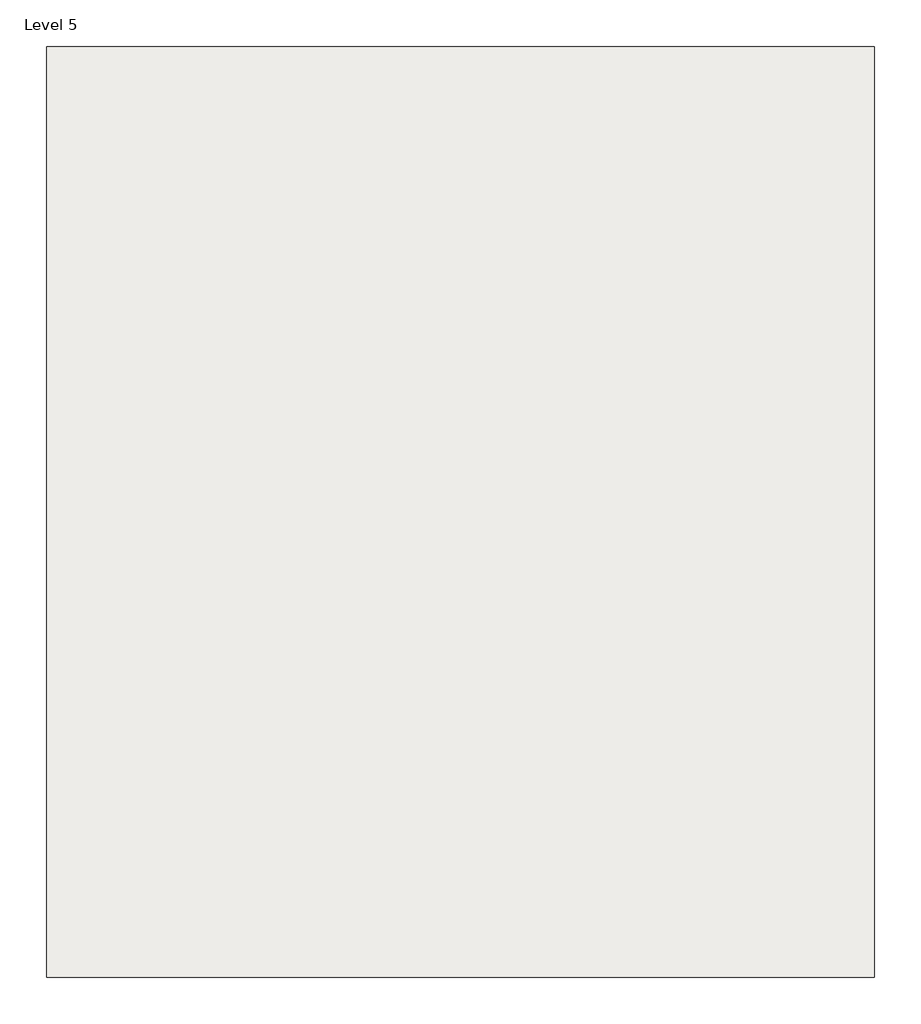
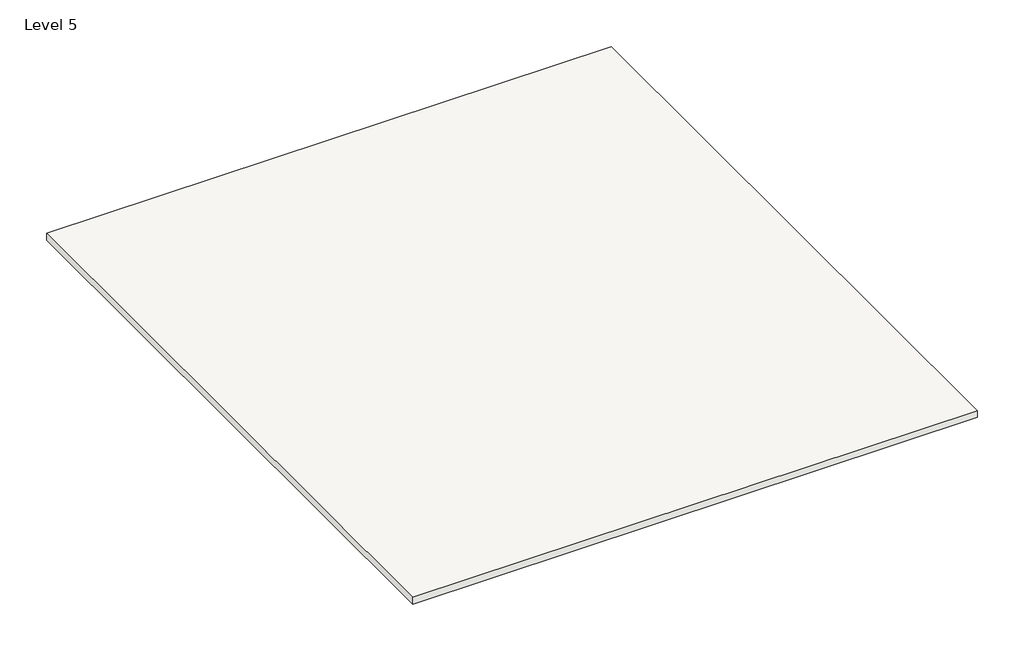
# One storey, incomplete: 1 roof.
"""IFC4 building model written with IfcOpenShell, lengths in millimetres."""

from ifc_helpers import new_model, si_unit, frame, origin, place, context, project, spatial, polyline, outline, extrude, element, save

model = new_model("IFC4")

# Units and contexts
model_context = context("Model", 3, world=origin())
ifc_project = project(units=[si_unit("LENGTHUNIT", "METRE", prefix="MILLI")], contexts=[model_context])

# Site, building, storey
site = spatial("IfcSite", under=ifc_project)
building = spatial("IfcBuilding", under=site)
storey = spatial("IfcBuildingStorey", under=building, Name="Level 5", Elevation=12192.0)

# Roof
placement = place(None, origin())
element("IfcRoof", 1, ObjectType="Generic - 12\"", at=placement, inside=storey, context=model_context, shape_type="SweptSolid", body=[
    extrude(outline(polyline([(-6906.5690281, 7421.1495467), (5272.7309719, 7421.1495467), (5272.7309719, -6269.4504533), (-6906.5690281, -6269.4504533), (-6906.5690281, 7421.1495467)])), frame((0.0, 0.0, 12192.0), z_axis=(0.0, 0.0, 1.0), x_axis=(1.0, 0.0, 0.0)), (0.0, 0.0, 1.0), 152.4),
])

save(model, "model.ifc")

# Revit data of these elements
# Type "Generic - 12\""
#   Assembly Code = "B1020"
#   Layers, outside or top first: 0' - 6" no material (function 1)
# Element 1 (IfcRoof, "Generic - 12\"")
#   built-in parameter 1001705 = 40.5 (stored number, unit not read)
#   built-in parameter 1001710 = 33615
#   Phase Created = New Construction
#   Materials on its faces: "Default Roof"
# Materials
#   "Default Roof": colour RGB 88 101 114, transparency 0, Cost = 0
